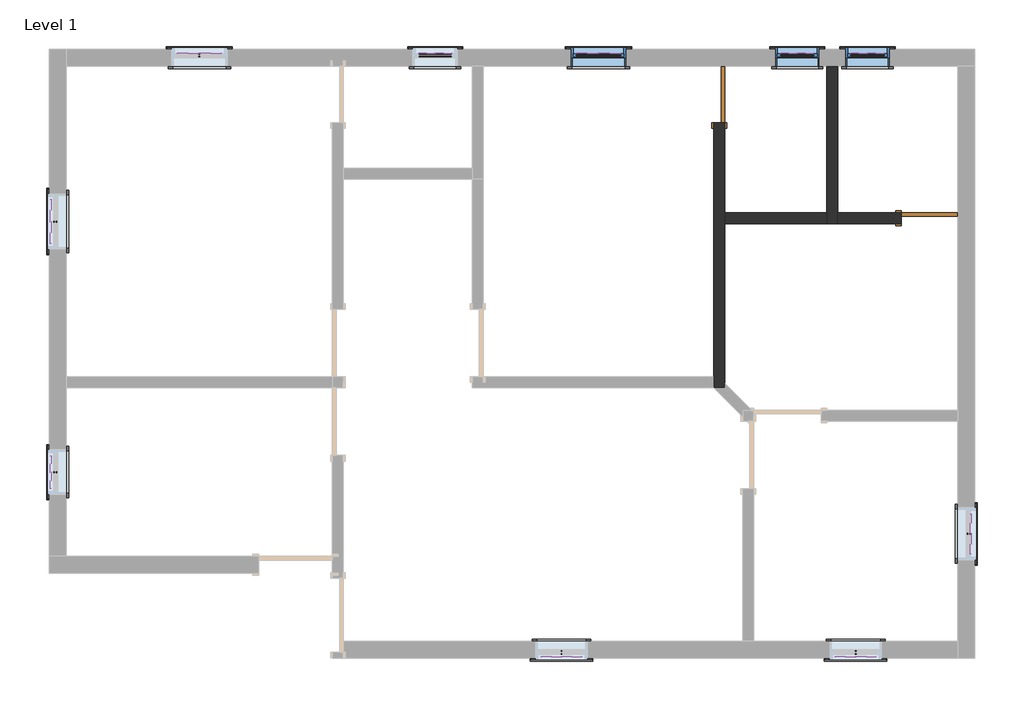
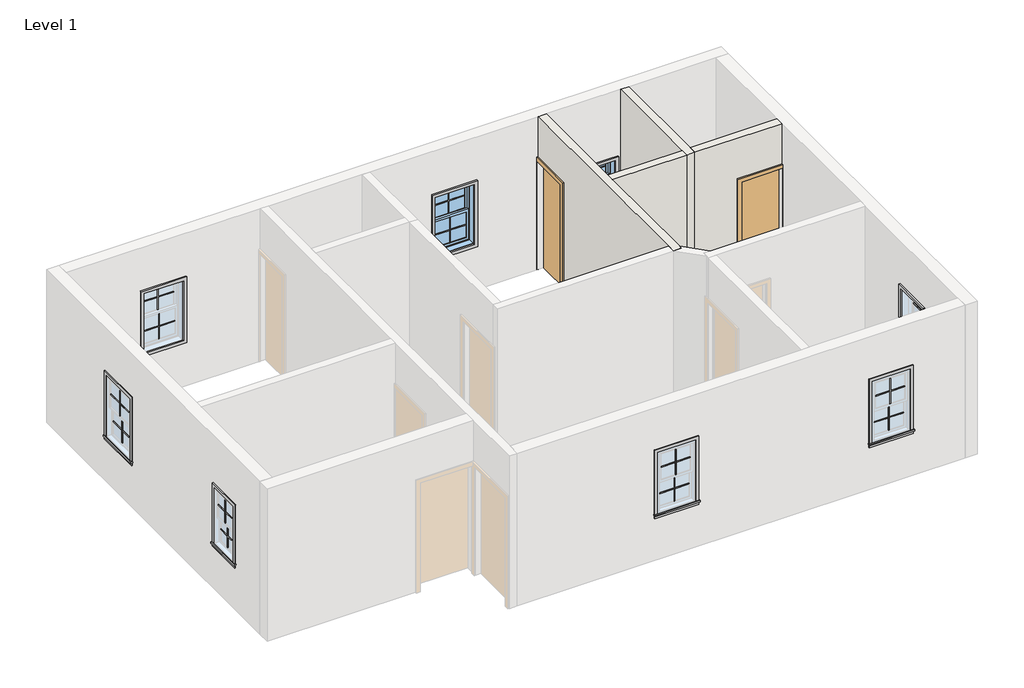
# One storey, part 2 of 2: 40 proxies, 4 walls, 3 windows, 2 doors.
"""IFC4 building model written with IfcOpenShell, lengths in millimetres."""

from ifc_helpers import new_model, si_unit, frame, origin, origin_with_axes, place, context, project, spatial, polyline, outline, extrude, faceted_brep, transform, mapped, element, save
from components import m_muntin_pattern_2x2_m_muntin_pattern_2x2_6483b455, m_muntin_pattern_2x2_m_muntin_pattern_2x2_aaec3afb, m_muntin_pattern_2x2_m_muntin_pattern_2x2_8c828626, m_muntin_pattern_2x2_m_muntin_pattern_2x2_b5651a11, m_trim_window_exterior_flat_with_sill_4c9fee41, m_trim_window_exterior_flat_with_sill_e7ff6350, m_trim_window_exterior_flat_with_sill_7a42a2ef, m_trim_window_exterior_flat_with_sill_a736bdd3, m_trim_window_interior_flat_picture_frame_87adca9b, m_trim_window_interior_flat_picture_frame_31bd2320, m_trim_window_interior_flat_picture_frame_c294611c, m_trim_window_interior_flat_picture_frame_c0d0133e, m_single_flush_0762_x_2134mm_8c18b9de, m_single_flush_0762_x_2134mm_1533e4c5, m_window_double_hung_600_x_750mm_49d140ec, m_window_double_hung_750_x_1200mm_abb80fbd

model = new_model("IFC4")

# Units and contexts
model_context = context("Model", 3, world=origin())
ifc_project = project(units=[si_unit("LENGTHUNIT", "METRE", prefix="MILLI")], contexts=[model_context])

# Site, building, storey
site = spatial("IfcSite", under=ifc_project)
building = spatial("IfcBuilding", under=site)
storey = spatial("IfcBuildingStorey", under=building, Name="Level 1", Elevation=0.0)

# Proxies
placement = place(None, origin())
m_muntin_pattern_2x2_m_muntin_pattern_2x2_shape = m_muntin_pattern_2x2_m_muntin_pattern_2x2_6483b455(model_context)
element("IfcBuildingElementProxy", 1, Name="M_Muntin Pattern_2x2 : M_Muntin Pattern_2x2", ObjectType="M_Muntin Pattern_2x2 : M_Muntin Pattern_2x2", at=placement, inside=storey, context=model_context, shape_type="MappedRepresentation", body=[
    mapped(m_muntin_pattern_2x2_m_muntin_pattern_2x2_shape, transform((5465.5587578, -19133.8303365, 1486.625), x_axis=(0.0, 1.0, 0.0), y_axis=(-1.0, 0.0, 0.0), z_axis=(0.0, 0.0, 1.0))),
])
element("IfcBuildingElementProxy", 2, Name="M_Muntin Pattern_2x2 : M_Muntin Pattern_2x2", ObjectType="M_Muntin Pattern_2x2 : M_Muntin Pattern_2x2", at=placement, inside=storey, context=model_context, shape_type="MappedRepresentation", body=[
    mapped(m_muntin_pattern_2x2_m_muntin_pattern_2x2_shape, transform((5510.0087578, -19133.8303365, 990.6), x_axis=(0.0, 1.0, 0.0), y_axis=(-1.0, 0.0, 0.0), z_axis=(0.0, 0.0, 1.0))),
])
m_muntin_pattern_2x2_m_muntin_pattern_2x2_2_shape = m_muntin_pattern_2x2_m_muntin_pattern_2x2_aaec3afb(model_context)
element("IfcBuildingElementProxy", 3, Name="M_Muntin Pattern_2x2 : M_Muntin Pattern_2x2", ObjectType="M_Muntin Pattern_2x2 : M_Muntin Pattern_2x2", at=placement, inside=storey, context=model_context, shape_type="MappedRepresentation", body=[
    mapped(m_muntin_pattern_2x2_m_muntin_pattern_2x2_2_shape, transform((5465.5587578, -15743.8303365, 1536.625), x_axis=(0.0, 1.0, 0.0), y_axis=(-1.0, 0.0, 0.0), z_axis=(0.0, 0.0, 1.0))),
])
element("IfcBuildingElementProxy", 4, Name="M_Muntin Pattern_2x2 : M_Muntin Pattern_2x2", ObjectType="M_Muntin Pattern_2x2 : M_Muntin Pattern_2x2", at=placement, inside=storey, context=model_context, shape_type="MappedRepresentation", body=[
    mapped(m_muntin_pattern_2x2_m_muntin_pattern_2x2_2_shape, transform((5510.0087578, -15743.8303365, 990.6), x_axis=(0.0, 1.0, 0.0), y_axis=(-1.0, 0.0, 0.0), z_axis=(0.0, 0.0, 1.0))),
])
element("IfcBuildingElementProxy", 5, Name="M_Muntin Pattern_2x2 : M_Muntin Pattern_2x2", ObjectType="M_Muntin Pattern_2x2 : M_Muntin Pattern_2x2", at=placement, inside=storey, context=model_context, shape_type="MappedRepresentation", body=[
    mapped(m_muntin_pattern_2x2_m_muntin_pattern_2x2_2_shape, transform((7460.6337578, -13448.7553365, 1536.625), x_axis=(1.0, 0.0, 0.0), y_axis=(0.0, 1.0, 0.0), z_axis=(0.0, 0.0, 1.0))),
])
element("IfcBuildingElementProxy", 6, Name="M_Muntin Pattern_2x2 : M_Muntin Pattern_2x2", ObjectType="M_Muntin Pattern_2x2 : M_Muntin Pattern_2x2", at=placement, inside=storey, context=model_context, shape_type="MappedRepresentation", body=[
    mapped(m_muntin_pattern_2x2_m_muntin_pattern_2x2_2_shape, transform((7460.6337578, -13493.2053365, 990.6), x_axis=(1.0, 0.0, 0.0), y_axis=(0.0, 1.0, 0.0), z_axis=(0.0, 0.0, 1.0))),
])
element("IfcBuildingElementProxy", 7, Name="M_Muntin Pattern_2x2 : M_Muntin Pattern_2x2", ObjectType="M_Muntin Pattern_2x2 : M_Muntin Pattern_2x2", at=placement, inside=storey, context=model_context, shape_type="MappedRepresentation", body=[
    mapped(m_muntin_pattern_2x2_m_muntin_pattern_2x2_2_shape, transform((12860.6337578, -13448.7553365, 1536.625), x_axis=(1.0, 0.0, 0.0), y_axis=(0.0, 1.0, 0.0), z_axis=(0.0, 0.0, 1.0))),
])
element("IfcBuildingElementProxy", 8, Name="M_Muntin Pattern_2x2 : M_Muntin Pattern_2x2", ObjectType="M_Muntin Pattern_2x2 : M_Muntin Pattern_2x2", at=placement, inside=storey, context=model_context, shape_type="MappedRepresentation", body=[
    mapped(m_muntin_pattern_2x2_m_muntin_pattern_2x2_2_shape, transform((12860.6337578, -13493.2053365, 990.6), x_axis=(1.0, 0.0, 0.0), y_axis=(0.0, 1.0, 0.0), z_axis=(0.0, 0.0, 1.0))),
])
m_muntin_pattern_2x2_m_muntin_pattern_2x2_3_shape = m_muntin_pattern_2x2_m_muntin_pattern_2x2_8c828626(model_context)
element("IfcBuildingElementProxy", 9, Name="M_Muntin Pattern_2x2 : M_Muntin Pattern_2x2", ObjectType="M_Muntin Pattern_2x2 : M_Muntin Pattern_2x2", at=placement, inside=storey, context=model_context, shape_type="MappedRepresentation", body=[
    mapped(m_muntin_pattern_2x2_m_muntin_pattern_2x2_3_shape, transform((12360.6337578, -21618.9053365, 1536.625), x_axis=(-1.0, 0.0, 0.0), y_axis=(0.0, -1.0, 0.0), z_axis=(0.0, 0.0, 1.0))),
])
element("IfcBuildingElementProxy", 10, Name="M_Muntin Pattern_2x2 : M_Muntin Pattern_2x2", ObjectType="M_Muntin Pattern_2x2 : M_Muntin Pattern_2x2", at=placement, inside=storey, context=model_context, shape_type="MappedRepresentation", body=[
    mapped(m_muntin_pattern_2x2_m_muntin_pattern_2x2_3_shape, transform((12360.6337578, -21574.4553365, 990.6), x_axis=(-1.0, 0.0, 0.0), y_axis=(0.0, -1.0, 0.0), z_axis=(0.0, 0.0, 1.0))),
])
element("IfcBuildingElementProxy", 11, Name="M_Muntin Pattern_2x2 : M_Muntin Pattern_2x2", ObjectType="M_Muntin Pattern_2x2 : M_Muntin Pattern_2x2", at=placement, inside=storey, context=model_context, shape_type="MappedRepresentation", body=[
    mapped(m_muntin_pattern_2x2_m_muntin_pattern_2x2_3_shape, transform((16340.6337578, -21618.9053365, 1536.625), x_axis=(-1.0, 0.0, 0.0), y_axis=(0.0, -1.0, 0.0), z_axis=(0.0, 0.0, 1.0))),
])
element("IfcBuildingElementProxy", 12, Name="M_Muntin Pattern_2x2 : M_Muntin Pattern_2x2", ObjectType="M_Muntin Pattern_2x2 : M_Muntin Pattern_2x2", at=placement, inside=storey, context=model_context, shape_type="MappedRepresentation", body=[
    mapped(m_muntin_pattern_2x2_m_muntin_pattern_2x2_3_shape, transform((16340.6337578, -21574.4553365, 990.6), x_axis=(-1.0, 0.0, 0.0), y_axis=(0.0, -1.0, 0.0), z_axis=(0.0, 0.0, 1.0))),
])
element("IfcBuildingElementProxy", 13, Name="M_Muntin Pattern_2x2 : M_Muntin Pattern_2x2", ObjectType="M_Muntin Pattern_2x2 : M_Muntin Pattern_2x2", at=placement, inside=storey, context=model_context, shape_type="MappedRepresentation", body=[
    mapped(m_muntin_pattern_2x2_m_muntin_pattern_2x2_3_shape, transform((17915.7087578, -19968.8303365, 1536.625), x_axis=(0.0, -1.0, 0.0), y_axis=(1.0, 0.0, 0.0), z_axis=(0.0, 0.0, 1.0))),
])
element("IfcBuildingElementProxy", 14, Name="M_Muntin Pattern_2x2 : M_Muntin Pattern_2x2", ObjectType="M_Muntin Pattern_2x2 : M_Muntin Pattern_2x2", at=placement, inside=storey, context=model_context, shape_type="MappedRepresentation", body=[
    mapped(m_muntin_pattern_2x2_m_muntin_pattern_2x2_3_shape, transform((17871.2587578, -19968.8303365, 990.6), x_axis=(0.0, -1.0, 0.0), y_axis=(1.0, 0.0, 0.0), z_axis=(0.0, 0.0, 1.0))),
])
m_muntin_pattern_2x2_m_muntin_pattern_2x2_4_shape = m_muntin_pattern_2x2_m_muntin_pattern_2x2_b5651a11(model_context)
element("IfcBuildingElementProxy", 15, Name="M_Muntin Pattern_2x2 : M_Muntin Pattern_2x2", ObjectType="M_Muntin Pattern_2x2 : M_Muntin Pattern_2x2", at=placement, inside=storey, context=model_context, shape_type="MappedRepresentation", body=[
    mapped(m_muntin_pattern_2x2_m_muntin_pattern_2x2_4_shape, transform((10650.6337578, -13448.7553365, 1311.625), x_axis=(1.0, 0.0, 0.0), y_axis=(0.0, 1.0, 0.0), z_axis=(0.0, 0.0, 1.0))),
])
element("IfcBuildingElementProxy", 16, Name="M_Muntin Pattern_2x2 : M_Muntin Pattern_2x2", ObjectType="M_Muntin Pattern_2x2 : M_Muntin Pattern_2x2", at=placement, inside=storey, context=model_context, shape_type="MappedRepresentation", body=[
    mapped(m_muntin_pattern_2x2_m_muntin_pattern_2x2_4_shape, transform((10650.6337578, -13493.2053365, 990.6), x_axis=(1.0, 0.0, 0.0), y_axis=(0.0, 1.0, 0.0), z_axis=(0.0, 0.0, 1.0))),
])
element("IfcBuildingElementProxy", 17, Name="M_Muntin Pattern_2x2 : M_Muntin Pattern_2x2", ObjectType="M_Muntin Pattern_2x2 : M_Muntin Pattern_2x2", at=placement, inside=storey, context=model_context, shape_type="MappedRepresentation", body=[
    mapped(m_muntin_pattern_2x2_m_muntin_pattern_2x2_4_shape, transform((15550.6337578, -13448.7553365, 1311.625), x_axis=(1.0, 0.0, 0.0), y_axis=(0.0, 1.0, 0.0), z_axis=(0.0, 0.0, 1.0))),
])
element("IfcBuildingElementProxy", 18, Name="M_Muntin Pattern_2x2 : M_Muntin Pattern_2x2", ObjectType="M_Muntin Pattern_2x2 : M_Muntin Pattern_2x2", at=placement, inside=storey, context=model_context, shape_type="MappedRepresentation", body=[
    mapped(m_muntin_pattern_2x2_m_muntin_pattern_2x2_4_shape, transform((15550.6337578, -13493.2053365, 990.6), x_axis=(1.0, 0.0, 0.0), y_axis=(0.0, 1.0, 0.0), z_axis=(0.0, 0.0, 1.0))),
])
element("IfcBuildingElementProxy", 19, Name="M_Muntin Pattern_2x2 : M_Muntin Pattern_2x2", ObjectType="M_Muntin Pattern_2x2 : M_Muntin Pattern_2x2", at=placement, inside=storey, context=model_context, shape_type="MappedRepresentation", body=[
    mapped(m_muntin_pattern_2x2_m_muntin_pattern_2x2_4_shape, transform((16500.6337578, -13448.7553365, 1311.625), x_axis=(1.0, 0.0, 0.0), y_axis=(0.0, 1.0, 0.0), z_axis=(0.0, 0.0, 1.0))),
])
element("IfcBuildingElementProxy", 20, Name="M_Muntin Pattern_2x2 : M_Muntin Pattern_2x2", ObjectType="M_Muntin Pattern_2x2 : M_Muntin Pattern_2x2", at=placement, inside=storey, context=model_context, shape_type="MappedRepresentation", body=[
    mapped(m_muntin_pattern_2x2_m_muntin_pattern_2x2_4_shape, transform((16500.6337578, -13493.2053365, 990.6), x_axis=(1.0, 0.0, 0.0), y_axis=(0.0, 1.0, 0.0), z_axis=(0.0, 0.0, 1.0))),
])
m_trim_window_exterior_flat_with_sill_shape = m_trim_window_exterior_flat_with_sill_4c9fee41(model_context)
element("IfcBuildingElementProxy", 21, Name="M_Trim-Window-Exterior-Flat : with Sill", ObjectType="M_Trim-Window-Exterior-Flat : with Sill", at=placement, inside=storey, context=model_context, shape_type="MappedRepresentation", body=[
    mapped(m_trim_window_exterior_flat_with_sill_shape, transform((5430.6337578, -19133.8303365, 2014.4), x_axis=(0.0, -1.0, 0.0), y_axis=(0.0, 0.0, 1.0), z_axis=(-1.0, 0.0, 0.0))),
])
m_trim_window_exterior_flat_with_sill_2_shape = m_trim_window_exterior_flat_with_sill_e7ff6350(model_context)
element("IfcBuildingElementProxy", 22, Name="M_Trim-Window-Exterior-Flat : with Sill", ObjectType="M_Trim-Window-Exterior-Flat : with Sill", at=placement, inside=storey, context=model_context, shape_type="MappedRepresentation", body=[
    mapped(m_trim_window_exterior_flat_with_sill_2_shape, transform((5430.6337578, -15743.8303365, 2114.4), x_axis=(0.0, -1.0, 0.0), y_axis=(0.0, 0.0, 1.0), z_axis=(-1.0, 0.0, 0.0))),
])
element("IfcBuildingElementProxy", 23, Name="M_Trim-Window-Exterior-Flat : with Sill", ObjectType="M_Trim-Window-Exterior-Flat : with Sill", at=placement, inside=storey, context=model_context, shape_type="MappedRepresentation", body=[
    mapped(m_trim_window_exterior_flat_with_sill_2_shape, transform((7460.6337578, -13413.8303365, 2114.4), x_axis=(-1.0, 0.0, 0.0), y_axis=(0.0, 0.0, 1.0), z_axis=(0.0, 1.0, 0.0))),
])
element("IfcBuildingElementProxy", 24, Name="M_Trim-Window-Exterior-Flat : with Sill", ObjectType="M_Trim-Window-Exterior-Flat : with Sill", at=placement, inside=storey, context=model_context, shape_type="MappedRepresentation", body=[
    mapped(m_trim_window_exterior_flat_with_sill_2_shape, transform((12860.6337578, -13413.8303365, 2114.4), x_axis=(-1.0, 0.0, 0.0), y_axis=(0.0, 0.0, 1.0), z_axis=(0.0, 1.0, 0.0))),
])
m_trim_window_exterior_flat_with_sill_3_shape = m_trim_window_exterior_flat_with_sill_7a42a2ef(model_context)
element("IfcBuildingElementProxy", 25, Name="M_Trim-Window-Exterior-Flat : with Sill", ObjectType="M_Trim-Window-Exterior-Flat : with Sill", at=placement, inside=storey, context=model_context, shape_type="MappedRepresentation", body=[
    mapped(m_trim_window_exterior_flat_with_sill_3_shape, transform((12360.6337578, -21653.8303365, 2114.4), x_axis=(1.0, 0.0, 0.0), y_axis=(0.0, 0.0, 1.0), z_axis=(0.0, -1.0, 0.0))),
])
element("IfcBuildingElementProxy", 26, Name="M_Trim-Window-Exterior-Flat : with Sill", ObjectType="M_Trim-Window-Exterior-Flat : with Sill", at=placement, inside=storey, context=model_context, shape_type="MappedRepresentation", body=[
    mapped(m_trim_window_exterior_flat_with_sill_3_shape, transform((16340.6337578, -21653.8303365, 2114.4), x_axis=(1.0, 0.0, 0.0), y_axis=(0.0, 0.0, 1.0), z_axis=(0.0, -1.0, 0.0))),
])
element("IfcBuildingElementProxy", 27, Name="M_Trim-Window-Exterior-Flat : with Sill", ObjectType="M_Trim-Window-Exterior-Flat : with Sill", at=placement, inside=storey, context=model_context, shape_type="MappedRepresentation", body=[
    mapped(m_trim_window_exterior_flat_with_sill_3_shape, transform((17950.6337578, -19968.8303365, 2114.4), x_axis=(0.0, 1.0, 0.0), y_axis=(0.0, 0.0, 1.0), z_axis=(1.0, 0.0, 0.0))),
])
m_trim_window_exterior_flat_with_sill_4_shape = m_trim_window_exterior_flat_with_sill_a736bdd3(model_context)
element("IfcBuildingElementProxy", 28, Name="M_Trim-Window-Exterior-Flat : with Sill", ObjectType="M_Trim-Window-Exterior-Flat : with Sill", at=placement, inside=storey, context=model_context, shape_type="MappedRepresentation", body=[
    mapped(m_trim_window_exterior_flat_with_sill_4_shape, transform((10650.6337578, -13413.8303365, 1664.4), x_axis=(-1.0, 0.0, 0.0), y_axis=(0.0, 0.0, 1.0), z_axis=(0.0, 1.0, 0.0))),
])
element("IfcBuildingElementProxy", 29, Name="M_Trim-Window-Exterior-Flat : with Sill", ObjectType="M_Trim-Window-Exterior-Flat : with Sill", at=placement, inside=storey, context=model_context, shape_type="MappedRepresentation", body=[
    mapped(m_trim_window_exterior_flat_with_sill_4_shape, transform((15550.6337578, -13413.8303365, 1664.4), x_axis=(-1.0, 0.0, 0.0), y_axis=(0.0, 0.0, 1.0), z_axis=(0.0, 1.0, 0.0))),
])
element("IfcBuildingElementProxy", 30, Name="M_Trim-Window-Exterior-Flat : with Sill", ObjectType="M_Trim-Window-Exterior-Flat : with Sill", at=placement, inside=storey, context=model_context, shape_type="MappedRepresentation", body=[
    mapped(m_trim_window_exterior_flat_with_sill_4_shape, transform((16500.6337578, -13413.8303365, 1664.4), x_axis=(-1.0, 0.0, 0.0), y_axis=(0.0, 0.0, 1.0), z_axis=(0.0, 1.0, 0.0))),
])
m_trim_window_interior_flat_picture_frame_shape = m_trim_window_interior_flat_picture_frame_87adca9b(model_context)
element("IfcBuildingElementProxy", 31, Name="M_Trim-Window-Interior-Flat : Picture Frame", ObjectType="M_Trim-Window-Interior-Flat : Picture Frame", at=placement, inside=storey, context=model_context, shape_type="MappedRepresentation", body=[
    mapped(m_trim_window_interior_flat_picture_frame_shape, transform((5660.6337578, -19133.8303365, 2014.4), x_axis=(0.0, 1.0, 0.0), y_axis=(0.0, 0.0, 1.0), z_axis=(1.0, 0.0, 0.0))),
])
m_trim_window_interior_flat_picture_frame_2_shape = m_trim_window_interior_flat_picture_frame_31bd2320(model_context)
element("IfcBuildingElementProxy", 32, Name="M_Trim-Window-Interior-Flat : Picture Frame", ObjectType="M_Trim-Window-Interior-Flat : Picture Frame", at=placement, inside=storey, context=model_context, shape_type="MappedRepresentation", body=[
    mapped(m_trim_window_interior_flat_picture_frame_2_shape, transform((5660.6337578, -15743.8303365, 2114.4), x_axis=(0.0, 1.0, 0.0), y_axis=(0.0, 0.0, 1.0), z_axis=(1.0, 0.0, 0.0))),
])
element("IfcBuildingElementProxy", 33, Name="M_Trim-Window-Interior-Flat : Picture Frame", ObjectType="M_Trim-Window-Interior-Flat : Picture Frame", at=placement, inside=storey, context=model_context, shape_type="MappedRepresentation", body=[
    mapped(m_trim_window_interior_flat_picture_frame_2_shape, transform((7460.6337578, -13643.8303365, 2114.4), x_axis=(1.0, 0.0, 0.0), y_axis=(0.0, 0.0, 1.0), z_axis=(0.0, -1.0, 0.0))),
])
element("IfcBuildingElementProxy", 34, Name="M_Trim-Window-Interior-Flat : Picture Frame", ObjectType="M_Trim-Window-Interior-Flat : Picture Frame", at=placement, inside=storey, context=model_context, shape_type="MappedRepresentation", body=[
    mapped(m_trim_window_interior_flat_picture_frame_2_shape, transform((12860.6337578, -13643.8303365, 2114.4), x_axis=(1.0, 0.0, 0.0), y_axis=(0.0, 0.0, 1.0), z_axis=(0.0, -1.0, 0.0))),
])
m_trim_window_interior_flat_picture_frame_3_shape = m_trim_window_interior_flat_picture_frame_c294611c(model_context)
element("IfcBuildingElementProxy", 35, Name="M_Trim-Window-Interior-Flat : Picture Frame", ObjectType="M_Trim-Window-Interior-Flat : Picture Frame", at=placement, inside=storey, context=model_context, shape_type="MappedRepresentation", body=[
    mapped(m_trim_window_interior_flat_picture_frame_3_shape, transform((12360.6337578, -21423.8303365, 2114.4), x_axis=(-1.0, 0.0, 0.0), y_axis=(0.0, 0.0, 1.0), z_axis=(0.0, 1.0, 0.0))),
])
element("IfcBuildingElementProxy", 36, Name="M_Trim-Window-Interior-Flat : Picture Frame", ObjectType="M_Trim-Window-Interior-Flat : Picture Frame", at=placement, inside=storey, context=model_context, shape_type="MappedRepresentation", body=[
    mapped(m_trim_window_interior_flat_picture_frame_3_shape, transform((16340.6337578, -21423.8303365, 2114.4), x_axis=(-1.0, 0.0, 0.0), y_axis=(0.0, 0.0, 1.0), z_axis=(0.0, 1.0, 0.0))),
])
element("IfcBuildingElementProxy", 37, Name="M_Trim-Window-Interior-Flat : Picture Frame", ObjectType="M_Trim-Window-Interior-Flat : Picture Frame", at=placement, inside=storey, context=model_context, shape_type="MappedRepresentation", body=[
    mapped(m_trim_window_interior_flat_picture_frame_3_shape, transform((17720.6337578, -19968.8303365, 2114.4), x_axis=(0.0, -1.0, 0.0), y_axis=(0.0, 0.0, 1.0), z_axis=(-1.0, 0.0, 0.0))),
])
m_trim_window_interior_flat_picture_frame_4_shape = m_trim_window_interior_flat_picture_frame_c0d0133e(model_context)
element("IfcBuildingElementProxy", 38, Name="M_Trim-Window-Interior-Flat : Picture Frame", ObjectType="M_Trim-Window-Interior-Flat : Picture Frame", at=placement, inside=storey, context=model_context, shape_type="MappedRepresentation", body=[
    mapped(m_trim_window_interior_flat_picture_frame_4_shape, transform((10650.6337578, -13643.8303365, 1664.4), x_axis=(1.0, 0.0, 0.0), y_axis=(0.0, 0.0, 1.0), z_axis=(0.0, -1.0, 0.0))),
])
element("IfcBuildingElementProxy", 39, Name="M_Trim-Window-Interior-Flat : Picture Frame", ObjectType="M_Trim-Window-Interior-Flat : Picture Frame", at=placement, inside=storey, context=model_context, shape_type="MappedRepresentation", body=[
    mapped(m_trim_window_interior_flat_picture_frame_4_shape, transform((15550.6337578, -13643.8303365, 1664.4), x_axis=(1.0, 0.0, 0.0), y_axis=(0.0, 0.0, 1.0), z_axis=(0.0, -1.0, 0.0))),
])
element("IfcBuildingElementProxy", 40, Name="M_Trim-Window-Interior-Flat : Picture Frame", ObjectType="M_Trim-Window-Interior-Flat : Picture Frame", at=placement, inside=storey, context=model_context, shape_type="MappedRepresentation", body=[
    mapped(m_trim_window_interior_flat_picture_frame_4_shape, transform((16500.6337578, -13643.8303365, 1664.4), x_axis=(1.0, 0.0, 0.0), y_axis=(0.0, 0.0, 1.0), z_axis=(0.0, -1.0, 0.0))),
])

# Doors
m_single_flush_0762_x_2134mm_shape = m_single_flush_0762_x_2134mm_8c18b9de(model_context)
element("IfcDoor", 41, ObjectType="M_Single-Flush : 0762 x 2134mm", at=placement, inside=storey, context=model_context, shape_type="MappedRepresentation", body=[
    mapped(m_single_flush_0762_x_2134mm_shape, transform((14495.6337578, -14024.8303365, 0.0), x_axis=(0.0, 1.0, 0.0), y_axis=(-1.0, 0.0, 0.0), z_axis=(0.0, 0.0, 1.0))),
])
m_single_flush_0762_x_2134mm_2_shape = m_single_flush_0762_x_2134mm_1533e4c5(model_context)
element("IfcDoor", 42, ObjectType="M_Single-Flush : 0762 x 2134mm", at=placement, inside=storey, context=model_context, shape_type="MappedRepresentation", body=[
    mapped(m_single_flush_0762_x_2134mm_2_shape, transform((17339.6337578, -15698.8303365, 0.0), x_axis=(1.0, 0.0, 0.0), y_axis=(0.0, 1.0, 0.0), z_axis=(0.0, 0.0, 1.0))),
])

# Walls
element("IfcWall", 43, ObjectType="Interior-150mm", at=placement, inside=storey, context=model_context, shape_type="Brep", body=[
    faceted_brep([(14420.6337578, -17993.8303365, 3000.0), (14420.6337578, -17843.8303365, 3000.0), (14420.6337578, -13643.8303365, 3000.0), (14420.6337578, -13643.8303365, 2134.0), (14420.6337578, -14405.8303365, 2134.0), (14420.6337578, -14405.8303365, 0.0), (14420.6337578, -17843.8303365, 0.0), (14420.6337578, -17993.8303365, 0.0), (14570.6337578, -13643.8303365, 3000.0), (14570.6337578, -15623.8303365, 3000.0), (14570.6337578, -15773.8303365, 3000.0), (14570.6337578, -17931.6983022, 3000.0), (14570.6337578, -17993.8303365, 3000.0), (14570.6337578, -17993.8303365, 0.0), (14570.6337578, -17931.6983022, 0.0), (14570.6337578, -15773.8303365, 0.0), (14570.6337578, -15623.8303365, 0.0), (14570.6337578, -14405.8303365, 0.0), (14570.6337578, -14405.8303365, 2134.0), (14570.6337578, -13643.8303365, 2134.0)], [[[0, 1, 2, 3, 4, 5, 6, 7]], [[8, 9, 10, 11, 12, 13, 14, 15, 16, 17, 18, 19]], [[13, 7, 6, 5, 17, 16, 15, 14]], [[2, 1, 0, 12, 11, 10, 9, 8]], [[2, 8, 19, 3]], [[0, 7, 13, 12]], [[18, 4, 3, 19]], [[4, 18, 17, 5]]]),
])
element("IfcWall", 44, ObjectType="Interior-150mm", at=placement, inside=storey, context=model_context, shape_type="Brep", body=[
    faceted_brep([(15950.6337578, -13643.8303365, 0.0), (15950.6337578, -15623.8303365, 0.0), (15950.6337578, -15773.8303365, 0.0), (15950.6337578, -15773.8303365, 3000.0), (15950.6337578, -15623.8303365, 3000.0), (15950.6337578, -13643.8303365, 3000.0), (16100.6337578, -13643.8303365, 0.0), (16100.6337578, -13643.8303365, 3000.0), (16100.6337578, -15623.8303365, 3000.0), (16100.6337578, -15773.8303365, 3000.0), (16100.6337578, -15773.8303365, 0.0), (16100.6337578, -15623.8303365, 0.0)], [[[0, 1, 2, 3, 4, 5]], [[6, 7, 8, 9, 10, 11]], [[2, 1, 0, 6, 11, 10]], [[5, 4, 3, 9, 8, 7]], [[0, 5, 7, 6]], [[3, 2, 10, 9]]]),
])
element("IfcWall", 45, ObjectType="Interior-150mm", at=placement, inside=storey, context=model_context, shape_type="SweptSolid", body=[
    extrude(outline(polyline([(14570.6337578, -15623.8303365), (15950.6337578, -15623.8303365), (15950.6337578, -15773.8303365), (14570.6337578, -15773.8303365), (14570.6337578, -15623.8303365)])), origin_with_axes(), (0.0, 0.0, 1.0), 3000.0),
])
element("IfcWall", 46, ObjectType="Interior-150mm", at=placement, inside=storey, context=model_context, shape_type="SweptSolid", body=[
    extrude(outline(polyline([(3000.0, 17720.6337578), (3000.0, 16100.6337578), (0.0, 16100.6337578), (0.0, 16958.6337578), (2134.0, 16958.6337578), (2134.0, 17720.6337578), (3000.0, 17720.6337578)])), frame((0.0, -15773.8303365, 0.0), z_axis=(0.0, 1.0, 0.0), x_axis=(0.0, 0.0, 1.0)), (0.0, 0.0, 1.0), 150.0),
])

# Windows
m_window_double_hung_600_x_750mm_shape = m_window_double_hung_600_x_750mm_49d140ec(model_context)
element("IfcWindow", 47, ObjectType="M_Window-Double-Hung : 600 x 750mm", at=placement, inside=storey, context=model_context, shape_type="MappedRepresentation", body=[
    mapped(m_window_double_hung_600_x_750mm_shape, transform((15550.6337578, -13528.8303365, 0.0), x_axis=(1.0, 0.0, 0.0), y_axis=(0.0, 1.0, 0.0), z_axis=(0.0, 0.0, 1.0))),
])
element("IfcWindow", 48, ObjectType="M_Window-Double-Hung : 600 x 750mm", at=placement, inside=storey, context=model_context, shape_type="MappedRepresentation", body=[
    mapped(m_window_double_hung_600_x_750mm_shape, transform((16500.6337578, -13528.8303365, 0.0), x_axis=(1.0, 0.0, 0.0), y_axis=(0.0, 1.0, 0.0), z_axis=(0.0, 0.0, 1.0))),
])
m_window_double_hung_750_x_1200mm_shape = m_window_double_hung_750_x_1200mm_abb80fbd(model_context)
element("IfcWindow", 49, ObjectType="M_Window-Double-Hung : 750 x 1200mm", at=placement, inside=storey, context=model_context, shape_type="MappedRepresentation", body=[
    mapped(m_window_double_hung_750_x_1200mm_shape, transform((12860.6337578, -13528.8303365, 0.0), x_axis=(1.0, 0.0, 0.0), y_axis=(0.0, 1.0, 0.0), z_axis=(0.0, 0.0, 1.0))),
])

save(model, "model.ifc")

# Revit data of these elements
# Type "M_Muntin Pattern_2x2 : M_Muntin Pattern_2x2"
#   Width [instance default] = 1.2 m
#   Thickness = 0.0127 m
#   Height [instance default] = 1.2 m
#   Distance = 0.01905 m
#   Interior Material [instance default] = none
#   Exterior Material [instance default] = none
#   Default Elevation = 0
# Type "M_Trim-Window-Exterior-Flat : with Sill"
#   Trim Width = 0.06 m
#   Trim Thickness_Picture Frame = 0.03 m
#   Trim Thickness_with Sill = 0.01905 m
#   Sill Thickness = 0.03 m
#   Opening Width [instance default] = 0.6 m
#   Opening Height [instance default] = 0.9 m
#   Default Elevation = 1.2 m
#   Sill = yes
#   Picture Frame = no
#   Trim Material [instance default] = none
# Type "M_Trim-Window-Interior-Flat : Picture Frame"
#   Trim Thickness_Picture Frame = 0.03 m
#   Trim Width = 0.06 m
#   Trim Thickness_with Sill = 0.02 m
#   Sill Thickness = 0.03 m
#   Opening Width [instance default] = 0.6 m
#   Opening Height [instance default] = 0.9 m
#   Default Elevation = 1.2 m
#   Sill = no
#   Picture Frame = yes
#   Trim Material [instance default] = none
# Type "M_Single-Flush : 0762 x 2134mm"
#   Type Mark = "26"
#   Construction Type Id = "MDOOR"
#   Analytic Construction = "Metal"
#   Thickness = 0.051 m
#   Thermal Resistance (R) = 0.270117 (m²·K)/W
#   Heat Transfer Coefficient (U) = 3.7021 W/(m²·K)
#   Height = 2.134 m
#   Trim Projection Ext = 0.025 m
#   Trim Projection Int = 0.025 m
#   Trim Width = 0.076 m
#   Width = 0.762 m
#   Define Thermal Properties by = 1
#   Define Thermal Properties by = 1
#   Door Material = Door - Panel
#   Frame Material = Door - Frame
#   Visual Light Transmittance = 0
#   Solar Heat Gain Coefficient = 0
#   Function = (empty or 0)
#   Wall Closure = (empty or 0)
# Type "Interior-150mm"
#   Layers, outside or top first: 0.15 m no material (function 1)
# Type "M_Window-Double-Hung : 600 x 750mm"
#   Type Mark = "V"
#   Fire Rating = "0.5h"
#   Construction Type Id = "DG-DR"
#   Assembly Code = "B2020100"
#   Analytic Construction = "Double glazing - domestic"
#   Wall Thickness [instance default] = 0.15 m
#   Window Inset [instance default] = 0 m
#   Visual Light Transmittance = 0.81
#   Thermal Resistance (R) = 0.319569 (m²·K)/W
#   Solar Heat Gain Coefficient = 0.76
#   Muntin Width = 0.4476 m
#   Muntin Height = 0.276575 m
#   Interior Wall Closure [instance default] = 0.0357 m
#   Rough Width = 0.615 m
#   Rough Height = 0.765 m
#   Frame Extension [instance default] = 0.03175 m
#   Exterior Wall Closure [instance default] = 0.0127 m
#   Extension Jamb [instance default] = 0.0357 m
#   Heat Transfer Coefficient (U) = 3.12929 W/(m²·K)
#   Height = 0.75 m
#   Width = 0.6 m
#   Top Muntin Visibility = yes
#   Indicator Visibility [instance default] = yes
#   Extension Jamb Visibility [instance default] = yes
#   Interior Trim Visibility [instance default] = yes
#   Exterior Trim Visibility [instance default] = yes
#   Define Thermal Properties by = 1
#   Bottom Muntin Visibility = yes
#   Muntin Pattern = M_Muntin Pattern_2x2 : M_Muntin Pattern_2x2
#   Interior Trim Material = Wood - Stained
#   Interior Trim = M_Trim-Window-Interior-Flat : Picture Frame
#   Exterior Trim Material = Clad - White
#   Exterior Trim = M_Trim-Window-Exterior-Flat : with Sill
#   Glass Panel Material = Glass
#   Exterior Frame Material = Clad - White
#   Interior Frame Material = Wood - Stained
#   Wall Closure = (empty or 0)
# Type "M_Window-Double-Hung : 750 x 1200mm"
#   Type Mark = "W2"
#   Fire Rating = "0.5h"
#   Construction Type Id = "DG-DR"
#   Assembly Code = "B2020100"
#   Analytic Construction = "Double glazing - domestic"
#   Wall Thickness [instance default] = 0.15 m
#   Window Inset [instance default] = 0 m
#   Visual Light Transmittance = 0.81
#   Thermal Resistance (R) = 0.319569 (m²·K)/W
#   Solar Heat Gain Coefficient = 0.76
#   Muntin Width = 0.5976 m
#   Muntin Height = 0.501575 m
#   Interior Wall Closure [instance default] = 0.0357 m
#   Rough Width = 0.765 m
#   Rough Height = 1.215 m
#   Frame Extension [instance default] = 0.03175 m
#   Exterior Wall Closure [instance default] = 0.0127 m
#   Extension Jamb [instance default] = 0.0357 m
#   Heat Transfer Coefficient (U) = 3.12929 W/(m²·K)
#   Height = 1.2 m
#   Width = 0.75 m
#   Define Thermal Properties by = 1
#   Top Muntin Visibility = yes
#   Indicator Visibility [instance default] = yes
#   Extension Jamb Visibility [instance default] = yes
#   Interior Trim Visibility [instance default] = yes
#   Exterior Trim Visibility [instance default] = yes
#   Define Thermal Properties by = 1
#   Bottom Muntin Visibility = yes
#   Muntin Pattern = M_Muntin Pattern_2x2 : M_Muntin Pattern_2x2
#   Interior Trim Material = Wood - Stained
#   Interior Trim = M_Trim-Window-Interior-Flat : Picture Frame
#   Exterior Trim Material = Clad - White
#   Exterior Trim = M_Trim-Window-Exterior-Flat : with Sill
#   Glass Panel Material = Glass
#   Exterior Frame Material = Clad - White
#   Interior Frame Material = Wood - Stained
#   Wall Closure = (empty or 0)
# Elements 1, 2 (IfcBuildingElementProxy, "M_Muntin Pattern_2x2 : M_Muntin Pattern_2x2")
#   Width = 0.4476 m
#   Height = 0.451575 m
#   Interior Material = Wood - Stained
#   Exterior Material = Clad - White
#   Phase Created = New Construction
#   Materials on its faces: "Clad - White", "Wood - Stained"
# Elements 3, 4, 5, 6, 7, 8 (IfcBuildingElementProxy, "M_Muntin Pattern_2x2 : M_Muntin Pattern_2x2")
#   Width = 0.5976 m
#   Height = 0.501575 m
#   Interior Material = Wood - Stained
#   Exterior Material = Clad - White
#   Phase Created = New Construction
#   Materials on its faces: "Clad - White", "Wood - Stained"
# Elements 9, 10, 11, 12, 13, 14 (IfcBuildingElementProxy, "M_Muntin Pattern_2x2 : M_Muntin Pattern_2x2")
#   Width = 0.5476 m
#   Height = 0.501575 m
#   Interior Material = Wood - Stained
#   Exterior Material = Clad - White
#   Phase Created = New Construction
#   Materials on its faces: "Clad - White", "Wood - Stained"
# Elements 15, 16, 17, 18, 19, 20 (IfcBuildingElementProxy, "M_Muntin Pattern_2x2 : M_Muntin Pattern_2x2")
#   Width = 0.4476 m
#   Height = 0.276575 m
#   Interior Material = Wood - Stained
#   Exterior Material = Clad - White
#   Phase Created = New Construction
#   Materials on its faces: "Clad - White", "Wood - Stained"
# Element 21 (IfcBuildingElementProxy, "M_Trim-Window-Exterior-Flat : with Sill")
#   Opening Width = 0.6 m
#   Opening Height = 1.1 m
#   Trim Material = Clad - White
#   Phase Created = New Construction
#   Materials on its faces: "Clad - White"
# Elements 22, 23, 24 (IfcBuildingElementProxy, "M_Trim-Window-Exterior-Flat : with Sill")
#   Opening Width = 0.75 m
#   Opening Height = 1.2 m
#   Trim Material = Clad - White
#   Phase Created = New Construction
#   Materials on its faces: "Clad - White"
# Elements 25, 26, 27 (IfcBuildingElementProxy, "M_Trim-Window-Exterior-Flat : with Sill")
#   Opening Width = 0.7 m
#   Opening Height = 1.2 m
#   Trim Material = Clad - White
#   Phase Created = New Construction
#   Materials on its faces: "Clad - White"
# Elements 28, 29, 30 (IfcBuildingElementProxy, "M_Trim-Window-Exterior-Flat : with Sill")
#   Opening Width = 0.6 m
#   Opening Height = 0.75 m
#   Trim Material = Clad - White
#   Phase Created = New Construction
#   Materials on its faces: "Clad - White"
# Element 31 (IfcBuildingElementProxy, "M_Trim-Window-Interior-Flat : Picture Frame")
#   Opening Width = 0.6 m
#   Opening Height = 1.1 m
#   Trim Material = Wood - Stained
#   Phase Created = New Construction
#   Materials on its faces: "Wood - Stained"
# Elements 32, 33, 34 (IfcBuildingElementProxy, "M_Trim-Window-Interior-Flat : Picture Frame")
#   Opening Width = 0.75 m
#   Opening Height = 1.2 m
#   Trim Material = Wood - Stained
#   Phase Created = New Construction
#   Materials on its faces: "Wood - Stained"
# Elements 35, 36, 37 (IfcBuildingElementProxy, "M_Trim-Window-Interior-Flat : Picture Frame")
#   Opening Width = 0.7 m
#   Opening Height = 1.2 m
#   Trim Material = Wood - Stained
#   Phase Created = New Construction
#   Materials on its faces: "Wood - Stained"
# Elements 38, 39, 40 (IfcBuildingElementProxy, "M_Trim-Window-Interior-Flat : Picture Frame")
#   Opening Width = 0.6 m
#   Opening Height = 0.75 m
#   Trim Material = Wood - Stained
#   Phase Created = New Construction
#   Materials on its faces: "Wood - Stained"
# Elements 41, 42 (IfcDoor, "M_Single-Flush : 0762 x 2134mm")
#   Phase Created = New Construction
#   Materials on its faces: "Door - Frame", "Door - Panel"
# Elements 43, 44, 45, 46 (IfcWall, "Interior-150mm")
#   Top Offset = 0 m
#   Base Offset = 0 m
#   wall height = 3 m
#   Phase Created = New Construction
#   Base Constraint = Level 1
#   Top Constraint = Level 2
#   Materials on its faces: "Default Wall"
# Element 47 (IfcWindow, "M_Window-Double-Hung : 600 x 750mm")
#   Mark = "12"
#   Window Inset = 0 m
#   Interior Wall Closure = 0.0357 m
#   Frame Extension = 0.03175 m
#   Exterior Wall Closure = 0.0127 m
#   Interior Trim Visibility = yes
#   Indicator Visibility = yes
#   Exterior Trim Visibility = yes
#   Phase Created = New Construction
#   Materials on its faces: "Wood - Stained", "Glass", "Clad - White"
# Element 48 (IfcWindow, "M_Window-Double-Hung : 600 x 750mm")
#   Mark = "13"
#   Window Inset = 0 m
#   Interior Wall Closure = 0.0357 m
#   Frame Extension = 0.03175 m
#   Exterior Wall Closure = 0.0127 m
#   Interior Trim Visibility = yes
#   Indicator Visibility = yes
#   Exterior Trim Visibility = yes
#   Phase Created = New Construction
#   Materials on its faces: "Wood - Stained", "Glass", "Clad - White"
# Element 49 (IfcWindow, "M_Window-Double-Hung : 750 x 1200mm")
#   Mark = "7"
#   Window Inset = 0 m
#   Interior Wall Closure = 0.0357 m
#   Frame Extension = 0.03175 m
#   Exterior Wall Closure = 0.0127 m
#   Interior Trim Visibility = yes
#   Indicator Visibility = yes
#   Exterior Trim Visibility = yes
#   Phase Created = New Construction
#   Materials on its faces: "Wood - Stained", "Glass", "Clad - White"
# Materials
#   "Door - Panel": class "Wood", colour RGB 210 159 95, transparency 0, Cost = 0
#   "Door - Frame": colour RGB 118 70 51, transparency 0, Cost = 0
#   "Wood - Stained": class "Wood", colour RGB 224 178 126, transparency 0, Cost = 0
#   "Clad - White": class "Wood", colour RGB 242 242 238, transparency 0, Cost = 0
#   "Glass": class "Glass", colour RGB 0 128 192, transparency 0.9, Description = "Soda Lime Glass", Cost = 0
#   "Default Wall": colour RGB 128 128 128, transparency 0, Cost = 0
